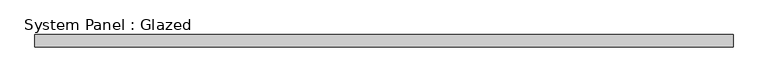
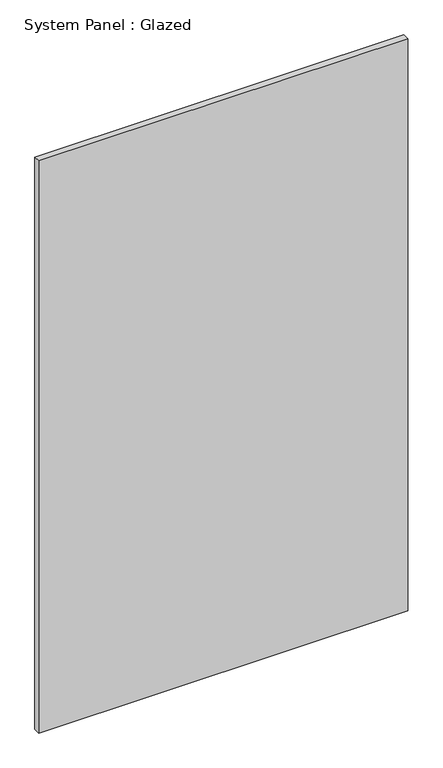
"""IFC4 building model written with IfcOpenShell, lengths in millimetres: plate geometry, System Panel : Glazed."""

from ifc_helpers import new_model, si_unit, origin, origin_with_axes, place, context, project, spatial, polyline, outline, extrude, source, transform, mapped, element, save


def system_panel_glazed_f9f53b74(model_context):
    return source(origin(), model_context, "Body", "SweptSolid", [
        extrude(outline(polyline([(714.3750001, 19.05), (-714.3750001, 19.05), (-714.3750001, 44.45), (714.3750001, 44.45), (714.3750001, 19.05)])), origin_with_axes(), (0.0, 0.0, 1.0), 2343.15),
    ])


if __name__ == "__main__":
    model = new_model("IFC4")
    model_context = context("Model", 3, world=origin())
    ifc_project = project(units=[si_unit("LENGTHUNIT", "METRE", prefix="MILLI")], contexts=[model_context])
    site = spatial("IfcSite", under=ifc_project)
    building = spatial("IfcBuilding", under=site)
    placement = place(None, origin())
    system_panel_glazed_shape = system_panel_glazed_f9f53b74(model_context)
    element("IfcPlate", 1, ObjectType="System Panel : Glazed", at=placement, inside=building, context=model_context, shape_type="MappedRepresentation", body=[
        mapped(system_panel_glazed_shape, transform((0.0, 0.0, 0.0), x_axis=(1.0, 0.0, 0.0), y_axis=(0.0, 1.0, 0.0), z_axis=(0.0, 0.0, 1.0))),
    ])
    save(model, "model.ifc")

# Revit data of these elements
# Type "System Panel : Glazed"
#   Construction Type Id = "GSP4R"
#   Analytic Construction = "1/8 in Pilkington single glazing"
#   Visual Light Transmittance = 0.9
#   Solar Heat Gain Coefficient = 0.86
#   Heat Transfer Coefficient (U) = 1.18115 BTU/(h·ft²·°F)
#   Define Thermal Properties by = 1
# Element 1 (IfcPlate, "System Panel : Glazed")
#   Materials on its faces: "Glass"
# Materials
#   "Glass": class "Glass", colour RGB 0 128 192, transparency 0.75, Description = "Soda Lime Glass", Cost = 0
